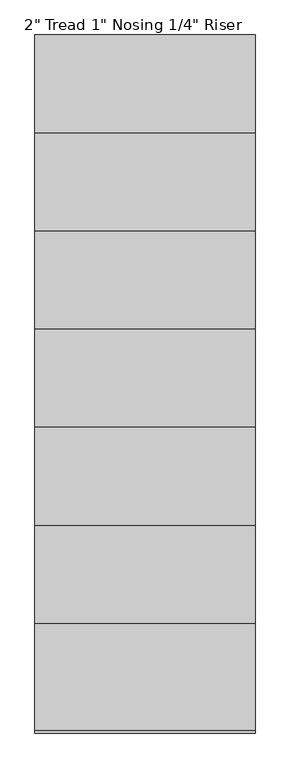
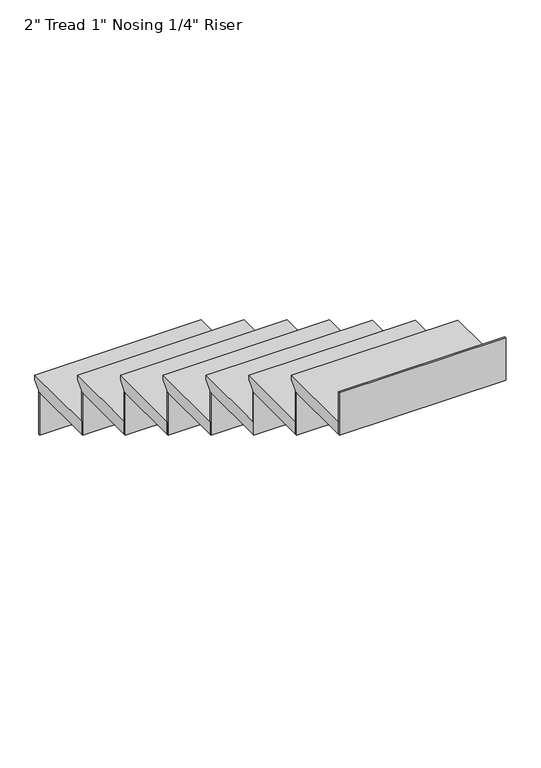
"""IFC4 building model written with IfcOpenShell, lengths in millimetres: stair flight geometry."""

from ifc_helpers import new_model, si_unit, frame, origin, place, context, project, spatial, polyline, outline, extrude, source, transform, mapped, element, save


def stair_flight_d75c07b6(model_context):
    return source(origin(), model_context, "Body", "SweptSolid", [
        extrude(outline(polyline([(8546.2516835, 1354.6666667), (8851.0516835, 1354.6666667), (8851.0516835, 1335.6166667), (8825.6516835, 1310.2166667), (8825.6516835, 1303.8666667), (8546.2516835, 1303.8666667), (8546.2516835, 1354.6666667)])), frame((-9169.9689718, 0.0, 0.0), z_axis=(1.0, 0.0, 0.0), x_axis=(0.0, 1.0, 0.0)), (0.0, 0.0, 1.0), 626.6396916),
        extrude(outline(polyline([(-9169.9689718, 8819.3016835), (-9169.9689718, 8825.6516835), (-8543.3292802, 8825.6516835), (-8543.3292802, 8819.3016835), (-9169.9689718, 8819.3016835)])), frame((0.0, 0.0, 1134.5333333), z_axis=(0.0, 0.0, 1.0), x_axis=(1.0, 0.0, 0.0)), (0.0, 0.0, 1.0), 169.3333333),
        extrude(outline(polyline([(-9169.9689718, 8539.9016835), (-9169.9689718, 8546.2516835), (-8543.3292802, 8546.2516835), (-8543.3292802, 8539.9016835), (-9169.9689718, 8539.9016835)])), frame((0.0, 0.0, 1303.8666667), z_axis=(0.0, 0.0, 1.0), x_axis=(1.0, 0.0, 0.0)), (0.0, 0.0, 1.0), 169.3333333),
        extrude(outline(polyline([(8266.8516835, 1524.0), (8571.6516835, 1524.0), (8571.6516835, 1504.95), (8546.2516835, 1479.55), (8546.2516835, 1473.2), (8266.8516835, 1473.2), (8266.8516835, 1524.0)])), frame((-9169.9689718, 0.0, 0.0), z_axis=(1.0, 0.0, 0.0), x_axis=(0.0, 1.0, 0.0)), (0.0, 0.0, 1.0), 626.6396916),
        extrude(outline(polyline([(-9169.9689718, 8260.5016835), (-9169.9689718, 8266.8516835), (-8543.3292802, 8266.8516835), (-8543.3292802, 8260.5016835), (-9169.9689718, 8260.5016835)])), frame((0.0, 0.0, 1473.2), z_axis=(0.0, 0.0, 1.0), x_axis=(1.0, 0.0, 0.0)), (0.0, 0.0, 1.0), 169.3333333),
        extrude(outline(polyline([(7987.4516835, 1693.3333333), (8292.2516835, 1693.3333333), (8292.2516835, 1674.2833333), (8266.8516835, 1648.8833333), (8266.8516835, 1642.5333333), (7987.4516835, 1642.5333333), (7987.4516835, 1693.3333333)])), frame((-9169.9689718, 0.0, 0.0), z_axis=(1.0, 0.0, 0.0), x_axis=(0.0, 1.0, 0.0)), (0.0, 0.0, 1.0), 626.6396916),
        extrude(outline(polyline([(-9169.9689718, 7981.1016835), (-9169.9689718, 7987.4516835), (-8543.3292802, 7987.4516835), (-8543.3292802, 7981.1016835), (-9169.9689718, 7981.1016835)])), frame((0.0, 0.0, 1642.5333333), z_axis=(0.0, 0.0, 1.0), x_axis=(1.0, 0.0, 0.0)), (0.0, 0.0, 1.0), 169.3333333),
        extrude(outline(polyline([(7708.0516835, 1862.6666667), (8012.8516835, 1862.6666667), (8012.8516835, 1843.6166667), (7987.4516835, 1818.2166667), (7987.4516835, 1811.8666667), (7708.0516835, 1811.8666667), (7708.0516835, 1862.6666667)])), frame((-9169.9689718, 0.0, 0.0), z_axis=(1.0, 0.0, 0.0), x_axis=(0.0, 1.0, 0.0)), (0.0, 0.0, 1.0), 626.6396916),
        extrude(outline(polyline([(-9169.9689718, 7701.7016835), (-9169.9689718, 7708.0516835), (-8543.3292802, 7708.0516835), (-8543.3292802, 7701.7016835), (-9169.9689718, 7701.7016835)])), frame((0.0, 0.0, 1811.8666667), z_axis=(0.0, 0.0, 1.0), x_axis=(1.0, 0.0, 0.0)), (0.0, 0.0, 1.0), 169.3333333),
        extrude(outline(polyline([(7428.6516835, 2032.0), (7733.4516835, 2032.0), (7733.4516835, 2012.95), (7708.0516835, 1987.55), (7708.0516835, 1981.2), (7428.6516835, 1981.2), (7428.6516835, 2032.0)])), frame((-9169.9689718, 0.0, 0.0), z_axis=(1.0, 0.0, 0.0), x_axis=(0.0, 1.0, 0.0)), (0.0, 0.0, 1.0), 626.6396916),
        extrude(outline(polyline([(-9169.9689718, 7422.3016835), (-9169.9689718, 7428.6516835), (-8543.3292802, 7428.6516835), (-8543.3292802, 7422.3016835), (-9169.9689718, 7422.3016835)])), frame((0.0, 0.0, 1981.2), z_axis=(0.0, 0.0, 1.0), x_axis=(1.0, 0.0, 0.0)), (0.0, 0.0, 1.0), 169.3333333),
        extrude(outline(polyline([(7149.2516835, 2201.3333333), (7454.0516835, 2201.3333333), (7454.0516835, 2182.2833333), (7428.6516835, 2156.8833333), (7428.6516835, 2150.5333333), (7149.2516835, 2150.5333333), (7149.2516835, 2201.3333333)])), frame((-9169.9689718, 0.0, 0.0), z_axis=(1.0, 0.0, 0.0), x_axis=(0.0, 1.0, 0.0)), (0.0, 0.0, 1.0), 626.6396916),
        extrude(outline(polyline([(-9169.9689718, 7142.9016835), (-9169.9689718, 7149.2516835), (-8543.3292802, 7149.2516835), (-8543.3292802, 7142.9016835), (-9169.9689718, 7142.9016835)])), frame((0.0, 0.0, 2150.5333333), z_axis=(0.0, 0.0, 1.0), x_axis=(1.0, 0.0, 0.0)), (0.0, 0.0, 1.0), 169.3333333),
        extrude(outline(polyline([(-9169.9689718, 6863.5016835), (-9169.9689718, 6869.8516835), (-8543.3292802, 6869.8516835), (-8543.3292802, 6863.5016835), (-9169.9689718, 6863.5016835)])), frame((0.0, 0.0, 2319.8666667), z_axis=(0.0, 0.0, 1.0), x_axis=(1.0, 0.0, 0.0)), (0.0, 0.0, 1.0), 169.3333333),
        extrude(outline(polyline([(6869.8516835, 2370.6666667), (7174.6516835, 2370.6666667), (7174.6516835, 2351.6166667), (7149.2516835, 2326.2166667), (7149.2516835, 2319.8666667), (6869.8516835, 2319.8666667), (6869.8516835, 2370.6666667)])), frame((-9169.9689718, 0.0, 0.0), z_axis=(1.0, 0.0, 0.0), x_axis=(0.0, 1.0, 0.0)), (0.0, 0.0, 1.0), 626.6396916),
    ])


if __name__ == "__main__":
    model = new_model("IFC4")
    model_context = context("Model", 3, world=origin())
    ifc_project = project(units=[si_unit("LENGTHUNIT", "METRE", prefix="MILLI")], contexts=[model_context])
    site = spatial("IfcSite", under=ifc_project)
    building = spatial("IfcBuilding", under=site)
    placement = place(None, origin())
    stair_flight_shape = stair_flight_d75c07b6(model_context)
    element("IfcStairFlight", 1, ObjectType="2\" Tread 1\" Nosing 1/4\" Riser", at=placement, inside=building, context=model_context, shape_type="MappedRepresentation", body=[
        mapped(stair_flight_shape, transform((0.0, 0.0, 0.0), x_axis=(1.0, 0.0, 0.0), y_axis=(0.0, 1.0, 0.0), z_axis=(0.0, 0.0, 1.0))),
    ])
    save(model, "model.ifc")
